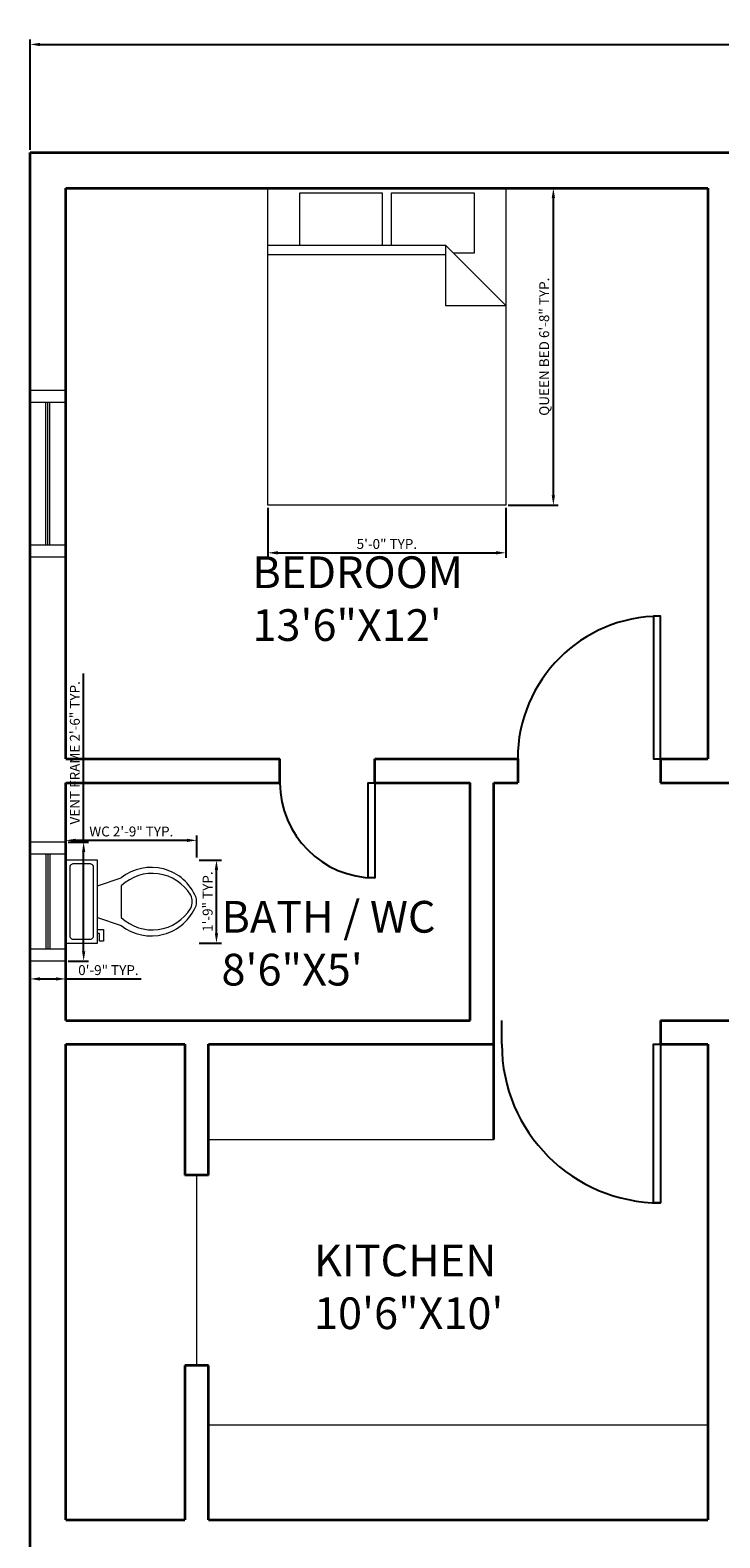
# Model space of a CAD drawing. Units: inches. Extents: x 2163 to 7246, y 928 to 2098.
# Tile 12 of 15: x 5233 to 5407, y 1651 to 2032. Entities that reach past the tile are written whole.
import ezdxf

# ---------------------------------------------------------------- set-up
doc = ezdxf.new("R2010")
doc.units = ezdxf.units.IN
for name, color, linetype, lineweight in [('A-ANNO-DIMS', 4, 'Continuous', 18), ('A-AREA-IDEN', 7, 'Continuous', 18), ('A-DOOR', 4, 'Continuous', 25), ('A-FLOR-FIXT', 9, 'Continuous', 20), ('A-FURN', 8, 'Continuous', 18), ('A-GLAZ', 30, 'Continuous', 20), ('A-WALL', 7, 'Continuous', 35)]:
    doc.layers.add(name, color=color, linetype=linetype, lineweight=lineweight)
doc.styles.get("Standard").update_dxf_attribs({"font": 'arial.ttf'})
doc.dimstyles.new('ISO-25', dxfattribs={"dimtxt": 2.5, "dimasz": 2.5, "dimexe": 1.25, "dimexo": 0.625, "dimtad": 1, "dimdec": 0, "dimlunit": 3, "dimtxsty": 'Standard', "dimcen": 2.5, "dimadec": 0, "dimazin": 0, "dimtfac": 1, "dimtdec": 0, "dimtmove": 0, "dimatfit": 3, "dimfxl": 1, "dimarcsym": 0})

# ---------------------------------------------------------------- blocks, each defined once
blk = doc.blocks.new('*U30')
for p, q in [((0, 0), (0, -6)), ((-36, 0), (-36, -6))]:
    blk.add_line(p, q)
blk.add_lwpolyline([(0, 0), (0, 36), (-1.75, 36), (-1.75, 0)], close=True)
blk.add_arc((0, 0), 36, 90, 180)
blk = doc.blocks.new('*U31')
for p, q in [((-24, 0), (-24, 6)), ((0, 0), (0, 6))]:
    blk.add_line(p, q)
blk.add_lwpolyline([(0, 0), (0, -24), (-1.75, -24), (-1.75, 0)], close=True)
blk.add_arc((0, 0), 24, 180, 270)
blk = doc.blocks.new('*U32')
for p, q in [((-40, 0), (-40, 6)), ((0, 0), (0, 6))]:
    blk.add_line(p, q)
blk.add_lwpolyline([(0, 0), (0, -40), (-1.75, -40), (-1.75, 0)], close=True)
blk.add_arc((0, 0), 40, 180, 270)
blk = doc.blocks.new('Bed - Queen')
for p, q in [((0, -80.00003), (0, 0)), ((0, 0), (59.99999, 0)), ((59.99999, 0), (59.99999, -80.00003)), ((7.99999, -1.2), (28.79998, -1.2)), ((7.99999, -14.4), (7.99999, -1.2)), ((28.79998, -1.2), (28.79998, -14.4)), ((31.19999, -1.2), (51.99999, -1.2)), ((31.19999, -14.4), (31.19999, -1.2)), ((51.99999, -1.2), (51.99999, -16.4)), ((0, -14.4), (44.8, -14.4)), ((59.99999, -29.6), (44.8, -14.4)), ((44.8, -14.4), (44.8, -29.6)), ((44.8, -16.8), (0, -16.8)), ((51.99999, -16.4), (46.79936, -16.4)), ((44.8, -29.6), (59.99999, -29.6)), ((59.99999, -80.00003), (0, -80.00003))]:
    blk.add_line(p, q)
blk = doc.blocks.new('Toilet - top')
for p, q in [((9.5, -6), (9.5, -2)), ((-10, -8.5), (-8, -8.5)), ((-10, -9.5), (-10, -8.5)), ((-7, -9.5), (-10, -9.5)), ((-8, -8.5), (-8, -8)), ((-7, -8), (-7, -9.5)), ((-4, -8), (-6, -14)), ((4, -8), (6, -14)), ((4, -14), (-4, -14))]:
    blk.add_line(p, q)
blk.add_lwpolyline([(10.5, -8), (10.5, 0), (-10.5, 0), (-10.5, -8)], close=True)
for points in [[(-9.5, -2), (-9.5, -6)], [(8.5, -1), (-8.5, -1)], [(-8.5, -7), (8.5, -7)]]:
    blk.add_lwpolyline(points)
for centre, radius, start, end in [((-8.62, -1.88), 0.884, 81.8699, 188.1301), ((8.62, -1.88), 0.884, 351.8699, 98.1301), ((-8.62, -6.12), 0.884, 171.8699, 278.1301), ((8.62, -6.12), 0.884, 261.8699, 8.1301), ((3.52, -21.58), 12.17, 141.4691, 247.9714), ((4.2, -21.82), 11.33, 136.3677, 238.9468), ((-3.52, -21.58), 12.17, 292.0284, 38.5307), ((-4.2, -21.82), 11.33, 301.053, 43.6321), ((0, -27.88), 4, 245.7318, 294.2682), ((0, -29), 4, 254.8605, 285.1395)]:
    blk.add_arc(centre, radius, start, end)
blk = doc.blocks.new('WIN-36-PLAN')
for p, q in [((0, 9), (0, 0)), ((3, 9), (3, 0)), ((39, 9), (39, 0)), ((42, 9), (42, 0)), ((3, 5), (39, 5)), ((3, 4.5), (39, 4.5)), ((3, 4), (39, 4))]:
    blk.add_line(p, q)
blk = doc.blocks.new('VENT-24-PLAN')
for p, q in [((9, 30), (0, 30)), ((9, 27), (0, 27)), ((4, 27), (4, 3)), ((4.5, 27), (4.5, 3)), ((5, 27), (5, 3)), ((9, 3), (0, 3)), ((9, 0), (0, 0))]:
    blk.add_line(p, q)
blk = doc.blocks.new('*D53')
at = {"layer": 'A-ANNO-DIMS', "color": 0, "lineweight": -2, "transparency": 16777216}
for p, q in [((5246.22, 1826.96), (5246.22, 1869.55)), ((5242.35, 1826.96), (5247.47, 1826.96)), ((5246.22, 1799.46), (5246.22, 1824.46)), ((5242.35, 1796.96), (5247.47, 1796.96))]:
    blk.add_line(p, q, dxfattribs=at)
at = {"layer": 'A-ANNO-DIMS', "color": 0, "transparency": 16777216}
for points in [[(5245.81, 1824.46), (5246.64, 1824.46), (5246.22, 1826.96)], [(5245.81, 1799.46), (5246.64, 1799.46), (5246.22, 1796.96)]]:
    blk.add_solid(points, dxfattribs=at)
at = {"layer": 'Defpoints', "color": 0, "transparency": 16777216}
for p in [(5241.72, 1826.96), (5246.22, 1826.96), (5241.72, 1796.96)]:
    blk.add_point(p, dxfattribs=at)
at = {"layer": 'A-ANNO-DIMS', "color": 0, "transparency": 16777216, "insert": (5244.32, 1849.5), "char_height": 2.5, "attachment_point": 5, "rotation": 90}
blk.add_mtext('VENT FRAME 2\'-6" TYP.', dxfattribs=at)
blk = doc.blocks.new('*D54')
at = {"layer": 'A-ANNO-DIMS', "color": 0, "lineweight": -2, "transparency": 16777216}
for p, q in [((5232.72, 1796.33), (5232.72, 1791.21)), ((5241.72, 1796.33), (5241.72, 1791.21)), ((5235.22, 1792.46), (5239.22, 1792.46)), ((5241.72, 1792.46), (5260.71, 1792.46))]:
    blk.add_line(p, q, dxfattribs=at)
at = {"layer": 'A-ANNO-DIMS', "color": 0, "transparency": 16777216}
for points in [[(5235.22, 1792.87), (5235.22, 1792.04), (5232.72, 1792.46)], [(5239.22, 1792.87), (5239.22, 1792.04), (5241.72, 1792.46)]]:
    blk.add_solid(points, dxfattribs=at)
at = {"layer": 'Defpoints', "color": 0, "transparency": 16777216}
for p in [(5232.72, 1796.96), (5241.72, 1796.96), (5241.72, 1792.46)]:
    blk.add_point(p, dxfattribs=at)
at = {"layer": 'A-ANNO-DIMS', "color": 0, "transparency": 16777216, "insert": (5252.47, 1794.36), "char_height": 2.5, "attachment_point": 5}
blk.add_mtext('0\'-9" TYP.', dxfattribs=at)
blk = doc.blocks.new('*D57')
at = {"layer": 'A-ANNO-DIMS', "color": 0, "lineweight": -2, "transparency": 16777216}
for p, q in [((5353.35, 1991.96), (5365.97, 1991.96)), ((5364.72, 1914.46), (5364.72, 1989.46)), ((5353.35, 1911.96), (5365.97, 1911.96))]:
    blk.add_line(p, q, dxfattribs=at)
at = {"layer": 'A-ANNO-DIMS', "color": 0, "transparency": 16777216}
for points in [[(5364.31, 1989.46), (5365.14, 1989.46), (5364.72, 1991.96)], [(5364.31, 1914.46), (5365.14, 1914.46), (5364.72, 1911.96)]]:
    blk.add_solid(points, dxfattribs=at)
at = {"layer": 'Defpoints', "color": 0, "transparency": 16777216}
for p in [(5352.72, 1991.96), (5364.72, 1991.96), (5352.72, 1911.96)]:
    blk.add_point(p, dxfattribs=at)
at = {"layer": 'A-ANNO-DIMS', "color": 0, "transparency": 16777216, "insert": (5362.73, 1951.96), "char_height": 2.5, "attachment_point": 5, "rotation": 90}
blk.add_mtext('QUEEN BED 6\'-8" TYP.', dxfattribs=at)
blk = doc.blocks.new('*D58')
at = {"layer": 'A-ANNO-DIMS', "color": 0, "lineweight": -2, "transparency": 16777216}
for p, q in [((5292.72, 1911.33), (5292.72, 1898.71)), ((5352.72, 1911.33), (5352.72, 1898.71)), ((5295.22, 1899.96), (5350.22, 1899.96))]:
    blk.add_line(p, q, dxfattribs=at)
at = {"layer": 'A-ANNO-DIMS', "color": 0, "transparency": 16777216}
for points in [[(5295.22, 1900.37), (5295.22, 1899.54), (5292.72, 1899.96)], [(5350.22, 1900.37), (5350.22, 1899.54), (5352.72, 1899.96)]]:
    blk.add_solid(points, dxfattribs=at)
at = {"layer": 'Defpoints', "color": 0, "transparency": 16777216}
for p in [(5292.72, 1911.96), (5352.72, 1911.96), (5352.72, 1899.96)]:
    blk.add_point(p, dxfattribs=at)
at = {"layer": 'A-ANNO-DIMS', "color": 0, "transparency": 16777216, "insert": (5322.72, 1901.86), "char_height": 2.5, "attachment_point": 5}
blk.add_mtext('5\'-0" TYP.', dxfattribs=at)
blk = doc.blocks.new('*D59')
at = {"layer": 'A-ANNO-DIMS', "color": 0, "lineweight": -2, "transparency": 16777216}
for p, q in [((5241.72, 1823.08), (5241.72, 1828.66)), ((5272.27, 1827.41), (5244.22, 1827.41)), ((5274.77, 1823.08), (5274.77, 1828.66))]:
    blk.add_line(p, q, dxfattribs=at)
at = {"layer": 'A-ANNO-DIMS', "color": 0, "transparency": 16777216}
for points in [[(5244.22, 1827.83), (5244.22, 1827), (5241.72, 1827.41)], [(5272.27, 1827.83), (5272.27, 1827), (5274.77, 1827.41)]]:
    blk.add_solid(points, dxfattribs=at)
at = {"layer": 'Defpoints', "color": 0, "transparency": 16777216}
for p in [(5241.72, 1827.41), (5241.72, 1822.46), (5274.77, 1822.46)]:
    blk.add_point(p, dxfattribs=at)
at = {"layer": 'A-ANNO-DIMS', "color": 0, "transparency": 16777216, "insert": (5258.25, 1829.33), "char_height": 2.5, "attachment_point": 5}
blk.add_mtext('WC 2\'-9" TYP.', dxfattribs=at)
blk = doc.blocks.new('*D60')
at = {"layer": 'A-ANNO-DIMS', "color": 0, "lineweight": -2, "transparency": 16777216}
for p, q in [((5275.39, 1822.46), (5280.98, 1822.46)), ((5279.73, 1803.96), (5279.73, 1819.96)), ((5275.39, 1801.46), (5280.98, 1801.46))]:
    blk.add_line(p, q, dxfattribs=at)
at = {"layer": 'A-ANNO-DIMS', "color": 0, "transparency": 16777216}
for points in [[(5279.31, 1819.96), (5280.14, 1819.96), (5279.73, 1822.46)], [(5279.31, 1803.96), (5280.14, 1803.96), (5279.73, 1801.46)]]:
    blk.add_solid(points, dxfattribs=at)
at = {"layer": 'Defpoints', "color": 0, "transparency": 16777216}
for p in [(5274.77, 1822.46), (5279.73, 1822.46), (5274.77, 1801.46)]:
    blk.add_point(p, dxfattribs=at)
at = {"layer": 'A-ANNO-DIMS', "color": 0, "transparency": 16777216, "insert": (5277.82, 1811.96), "char_height": 2.5, "attachment_point": 5, "rotation": 90}
blk.add_mtext('1\'-9" TYP.', dxfattribs=at)
blk = doc.blocks.new('*D109')
at = {"layer": 'A-ANNO-DIMS', "color": 0, "lineweight": -2, "transparency": 16777216}
for p, q in [((5232.72, 2001.58), (5232.72, 2029.46)), ((5235.22, 2028.21), (5602.22, 2028.21)), ((5604.72, 2001.58), (5604.72, 2029.46))]:
    blk.add_line(p, q, dxfattribs=at)
at = {"layer": 'A-ANNO-DIMS', "color": 0, "transparency": 16777216}
for points in [[(5235.22, 2028.62), (5235.22, 2027.79), (5232.72, 2028.21)], [(5602.22, 2028.62), (5602.22, 2027.79), (5604.72, 2028.21)]]:
    blk.add_solid(points, dxfattribs=at)
at = {"layer": 'Defpoints', "color": 0, "transparency": 16777216}
for p in [(5604.72, 2028.21), (5232.72, 2000.96), (5604.72, 2000.96)]:
    blk.add_point(p, dxfattribs=at)
at = {"layer": 'A-ANNO-DIMS', "color": 0, "transparency": 16777216, "insert": (5418.72, 2030.11), "char_height": 2.5, "attachment_point": 5}
blk.add_mtext('31\'-0"', dxfattribs=at)

msp = doc.modelspace()

# ---------------------------------------------------------------- linework, layer by layer
at = {"layer": 'A-FLOR-FIXT'}
for p, q in [((5277.72, 1751.96), (5349.72, 1751.96)), ((5277.72, 1679.96), (5403.72, 1679.96))]:
    msp.add_line(p, q, dxfattribs=at)
at = {"layer": 'A-GLAZ'}
msp.add_line((5274.72, 1742.96), (5274.72, 1694.96), dxfattribs=at)
at = {"layer": 'A-WALL'}
for p, q in [((5232.72, 2000.96), (5604.72, 2000.96)), ((5232.72, 1559.96), (5232.72, 2000.96)), ((5241.72, 1991.96), (5403.72, 1991.96)), ((5241.72, 1847.96), (5241.72, 1991.96)), ((5403.72, 1991.96), (5403.72, 1847.96)), ((5241.72, 1847.96), (5295.72, 1847.96)), ((5295.72, 1841.96), (5295.72, 1847.96)), ((5319.72, 1841.96), (5319.72, 1847.96)), ((5319.72, 1847.96), (5355.72, 1847.96)), ((5355.72, 1847.96), (5355.72, 1841.96)), ((5391.72, 1847.96), (5391.72, 1841.96)), ((5391.72, 1847.96), (5403.72, 1847.96)), ((5241.72, 1841.96), (5295.72, 1841.96)), ((5241.72, 1781.96), (5241.72, 1841.96)), ((5319.72, 1841.96), (5343.72, 1841.96)), ((5343.72, 1781.96), (5343.72, 1841.96)), ((5349.72, 1751.96), (5349.72, 1841.96)), ((5349.72, 1841.96), (5355.72, 1841.96)), ((5391.72, 1841.96), (5409.72, 1841.96)), ((5241.72, 1781.96), (5343.72, 1781.96)), ((5391.72, 1781.96), (5391.72, 1775.96)), ((5391.72, 1781.96), (5409.72, 1781.96)), ((5241.72, 1775.96), (5271.72, 1775.96)), ((5241.72, 1655.96), (5241.72, 1775.96)), ((5271.72, 1775.96), (5271.72, 1742.96)), ((5277.72, 1742.96), (5277.72, 1775.96)), ((5277.72, 1775.96), (5349.72, 1775.96)), ((5391.72, 1775.96), (5403.72, 1775.96)), ((5403.72, 1775.96), (5403.72, 1655.96)), ((5277.72, 1742.96), (5271.72, 1742.96)), ((5277.72, 1694.96), (5271.72, 1694.96)), ((5277.72, 1694.96), (5271.72, 1694.96)), ((5271.72, 1694.96), (5271.72, 1655.96)), ((5277.72, 1655.96), (5277.72, 1694.96)), ((5241.72, 1655.96), (5271.72, 1655.96)), ((5277.72, 1655.96), (5403.72, 1655.96))]:
    msp.add_line(p, q, dxfattribs=at)

# ---------------------------------------------------------------- block references
at = {"layer": 'A-DOOR'}
for name, p in [('*U30', (5391.72, 1847.96)), ('*U31', (5319.72, 1841.96)), ('*U32', (5391.72, 1775.96))]:
    msp.add_blockref(name, p, dxfattribs=at)
at = {"layer": 'A-FLOR-FIXT', "rotation": 90}
msp.add_blockref('Toilet - top', (5241.72, 1811.96), dxfattribs=at)
at = {"layer": 'A-FURN'}
msp.add_blockref('Bed - Queen', (5292.72, 1991.96), dxfattribs=at)
at = {"layer": 'A-GLAZ', "rotation": 90}
msp.add_blockref('WIN-36-PLAN', (5241.72, 1898.96), dxfattribs=at)
at = {"layer": 'A-GLAZ'}
msp.add_blockref('VENT-24-PLAN', (5232.72, 1796.96), dxfattribs=at)

# ---------------------------------------------------------------- texts
at = {"layer": 'A-AREA-IDEN', "char_height": 8, "attachment_point": 1}
for s, width, insert in [('BEDROOM\\P13\'6"X12\'', 462.4335, (5288.8, 1899.06)), ('BATH / WC\\P8\'6"X5\'', 344.4804, (5280.99, 1812.13)), ('KITCHEN\\P10\'6"X10\'', 70.9924, (5304.34, 1725.45))]:
    msp.add_mtext_dynamic_manual_height_columns(s, width=width, gutter_width=12.5, heights=[0], dxfattribs=dict(at, insert=insert))

# ---------------------------------------------------------------- dimensions: what is measured, and where the dimension line sits
at = {"layer": 'A-ANNO-DIMS'}
dim = msp.add_linear_dim(base=(5604.72, 2028.21), p1=(5232.72, 2000.96), p2=(5604.72, 2000.96), dimstyle='ISO-25', override={"dimdec": 1, "dimlfac": 1, "dimrnd": 0, "dimzin": 1, "dimdsep": 46, "dimlunit": 4, "dimfrac": 2}, dxfattribs=at)
dim.commit()
dim.dimension.update_dxf_attribs({"geometry": '*D109', "text_midpoint": (5418.72, 2030.11)})
for base, p1, p2, angle, text, picture, middle in [((5364.72, 1991.96), (5352.72, 1911.96), (5352.72, 1991.96), 90, 'QUEEN BED <> TYP.', '*D57', (5362.73, 1951.96)), ((5246.22, 1826.96), (5241.72, 1796.96), (5241.72, 1826.96), 90, 'VENT FRAME <> TYP.', '*D53', (5244.32, 1849.5)), ((5241.7231, 1827.413), (5274.7693, 1822.4561), (5241.7231, 1822.4561), 180, 'WC <> TYP.', '*D59', (5258.2462, 1829.3306)), ((5279.73, 1822.46), (5274.77, 1801.46), (5274.77, 1822.46), 90, '<> TYP.', '*D60', (5277.82, 1811.96))]:
    dim = msp.add_linear_dim(base=base, p1=p1, p2=p2, angle=angle, text=text, dimstyle='ISO-25', override={"dimdec": 1, "dimlfac": 1, "dimrnd": 0, "dimzin": 1, "dimdsep": 46, "dimlunit": 4, "dimfrac": 2}, dxfattribs=at)
    dim.commit()
    dim.dimension.update_dxf_attribs({"geometry": picture, "text_midpoint": middle})
for base, p1, p2, picture, middle in [((5352.72, 1899.96), (5292.72, 1911.96), (5352.72, 1911.96), '*D58', (5322.72, 1901.86)), ((5241.72, 1792.46), (5232.72, 1796.96), (5241.72, 1796.96), '*D54', (5252.47, 1794.36))]:
    dim = msp.add_linear_dim(base=base, p1=p1, p2=p2, text='<> TYP.', dimstyle='ISO-25', override={"dimdec": 1, "dimlfac": 1, "dimrnd": 0, "dimzin": 1, "dimdsep": 46, "dimlunit": 4, "dimfrac": 2}, dxfattribs=at)
    dim.commit()
    dim.dimension.update_dxf_attribs({"geometry": picture, "text_midpoint": middle})

doc.saveas('drawing.dxf')
